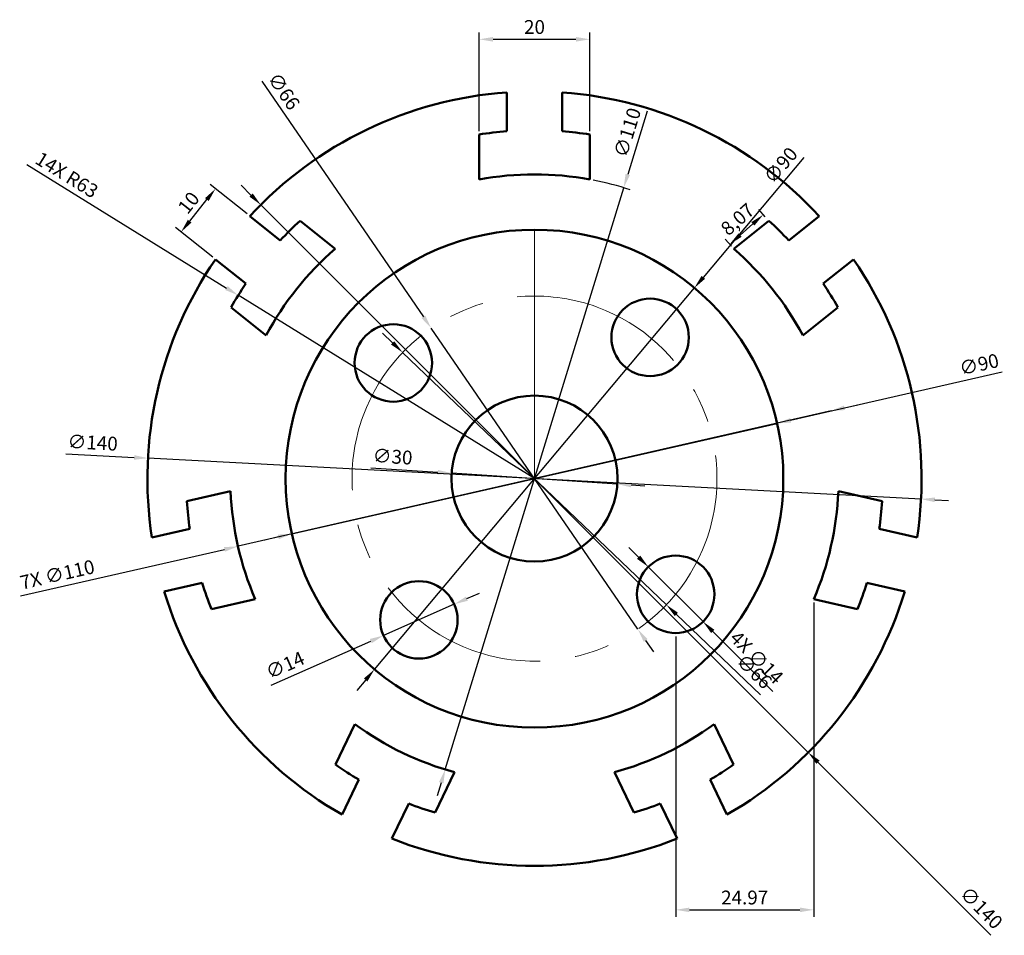
# Model space of a CAD drawing. Units: millimetres. Extents: x 3298 to 3476, y 1660 to 1825.
import ezdxf

# ---------------------------------------------------------------- set-up
doc = ezdxf.new("R2010")
doc.units = ezdxf.units.MM
doc.linetypes.add('CENTER', pattern=[50.8, 31.75, -6.35, 6.35, -6.35])
for name, color, linetype, lineweight in [('M-CNTR', 1, 'CENTER', 18), ('M-CONS', 8, 'Continuous', 13), ('M-DIMS', 2, 'Continuous', 25), ('M-OUTL', 7, 'Continuous', 50)]:
    doc.layers.add(name, color=color, linetype=linetype, lineweight=lineweight)
doc.styles.get("Standard").update_dxf_attribs({"font": 'arial.ttf'})
doc.dimstyles.new('ISO-25', dxfattribs={"dimtxt": 2.5, "dimasz": 2.5, "dimexe": 1.25, "dimexo": 0.625, "dimtad": 1, "dimtxsty": 'Standard', "dimcen": 2.5, "dimadec": 0, "dimazin": 0, "dimtfac": 1, "dimtmove": 0, "dimatfit": 3, "dimfxl": 1, "dimarcsym": 0})

# ---------------------------------------------------------------- blocks, each defined once
blk = doc.blocks.new('*D1')
at = {"layer": 'Defpoints', "color": 0, "transparency": 16777216}
for p in [(3375.77, 1743.34), (3405.71, 1741.37)]:
    blk.add_point(p, dxfattribs=at)
at = {"layer": 'M-DIMS', "color": 0, "lineweight": -2, "transparency": 16777216}
for p, q in [((3361.16, 1744.3), (3373.28, 1743.5)), ((3405.71, 1741.37), (3375.77, 1743.34)), ((3408.2, 1741.21), (3410.69, 1741.05))]:
    blk.add_line(p, q, dxfattribs=at)
at = {"layer": 'M-DIMS', "color": 0, "transparency": 16777216}
for points in [[(3373.3, 1743.92), (3373.25, 1743.09), (3375.77, 1743.34)], [(3408.23, 1741.62), (3408.17, 1740.79), (3405.71, 1741.37)]]:
    blk.add_solid(points, dxfattribs=at)
at = {"layer": 'M-DIMS', "color": 0, "transparency": 16777216, "insert": (3365.06, 1746.02), "char_height": 2.5, "attachment_point": 5, "rotation": 356.242}
blk.add_mtext('∅30', dxfattribs=at)
blk = doc.blocks.new('*D2')
at = {"layer": 'Defpoints', "color": 0, "transparency": 16777216}
for p in [(3434.62, 1752.34), (3346.86, 1732.37)]:
    blk.add_point(p, dxfattribs=at)
at = {"layer": 'M-DIMS', "color": 0, "lineweight": -2, "transparency": 16777216}
for p, q in [((3475.32, 1761.6), (3437.05, 1752.89)), ((3346.86, 1732.37), (3434.62, 1752.34)), ((3344.42, 1731.82), (3341.98, 1731.26))]:
    blk.add_line(p, q, dxfattribs=at)
at = {"layer": 'M-DIMS', "color": 0, "transparency": 16777216}
for points in [[(3436.96, 1753.3), (3437.15, 1752.49), (3434.62, 1752.34)], [(3344.33, 1732.23), (3344.51, 1731.41), (3346.86, 1732.37)]]:
    blk.add_solid(points, dxfattribs=at)
at = {"layer": 'M-DIMS', "color": 0, "transparency": 16777216, "insert": (3471.21, 1762.69), "char_height": 2.5, "attachment_point": 5, "rotation": 12.8166}
blk.add_mtext('∅90', dxfattribs=at)
blk = doc.blocks.new('*D3')
at = {"layer": 'Defpoints', "color": 0, "transparency": 16777216}
for p in [(3376.23, 1719.65), (3363.43, 1714)]:
    blk.add_point(p, dxfattribs=at)
at = {"layer": 'M-DIMS', "color": 0, "lineweight": -2, "transparency": 16777216}
for p, q in [((3378.52, 1720.66), (3380.81, 1721.67)), ((3376.23, 1719.65), (3363.43, 1714)), ((3343.11, 1705.03), (3361.14, 1712.99))]:
    blk.add_line(p, q, dxfattribs=at)
at = {"layer": 'M-DIMS', "color": 0, "transparency": 16777216}
for points in [[(3378.35, 1721.04), (3378.69, 1720.28), (3376.23, 1719.65)], [(3360.97, 1713.37), (3361.31, 1712.61), (3363.43, 1714)]]:
    blk.add_solid(points, dxfattribs=at)
at = {"layer": 'M-DIMS', "color": 0, "transparency": 16777216, "insert": (3345.77, 1708.36), "char_height": 2.5, "attachment_point": 5, "rotation": 23.8194}
blk.add_mtext('∅14', dxfattribs=at)
blk = doc.blocks.new('*D4')
at = {"layer": 'Defpoints', "color": 0, "transparency": 16777216}
for p in [(3372.05, 1769.56), (3409.42, 1715.15)]:
    blk.add_point(p, dxfattribs=at)
at = {"layer": 'M-DIMS', "color": 0, "lineweight": -2, "transparency": 16777216}
for p, q in [((3341.4, 1814.19), (3370.64, 1771.62)), ((3409.42, 1715.15), (3372.05, 1769.56)), ((3410.84, 1713.09), (3412.25, 1711.03))]:
    blk.add_line(p, q, dxfattribs=at)
at = {"layer": 'M-DIMS', "color": 0, "transparency": 16777216}
for points in [[(3370.98, 1771.85), (3370.3, 1771.38), (3372.05, 1769.56)], [(3411.18, 1713.33), (3410.49, 1712.86), (3409.42, 1715.15)]]:
    blk.add_solid(points, dxfattribs=at)
at = {"layer": 'M-DIMS', "color": 0, "transparency": 16777216, "insert": (3345.16, 1812.2), "char_height": 2.5, "attachment_point": 5, "rotation": 304.4835}
blk.add_mtext('∅66', dxfattribs=at)
blk = doc.blocks.new('*D5')
at = {"layer": 'Defpoints', "color": 0, "transparency": 16777216}
for p in [(3406.87, 1794.94), (3374.6, 1689.78)]:
    blk.add_point(p, dxfattribs=at)
at = {"layer": 'M-DIMS', "color": 0, "lineweight": -2, "transparency": 16777216}
for p, q in [((3411.12, 1808.78), (3407.61, 1797.33)), ((3374.6, 1689.78), (3406.87, 1794.94)), ((3373.87, 1687.39), (3373.14, 1685))]:
    blk.add_line(p, q, dxfattribs=at)
blk.add_arc((3390.74, 1742.36), 55, 71.6386, 78.8732, dxfattribs=at)
at = {"layer": 'M-DIMS', "color": 0, "transparency": 16777216}
for points in [[(3407.21, 1797.45), (3408, 1797.2), (3406.87, 1794.94)], [(3373.47, 1687.51), (3374.27, 1687.26), (3374.6, 1689.78)]]:
    blk.add_solid(points, dxfattribs=at)
at = {"layer": 'M-DIMS', "color": 0, "transparency": 16777216, "insert": (3407.85, 1804.83), "char_height": 2.5, "attachment_point": 5, "rotation": 72.9408}
blk.add_mtext('∅110', dxfattribs=at)
blk = doc.blocks.new('*D6')
at = {"layer": 'Defpoints', "color": 0, "transparency": 16777216}
for p in [(3400.74, 1821.77), (3380.74, 1804.56), (3400.74, 1804.56)]:
    blk.add_point(p, dxfattribs=at)
at = {"layer": 'M-DIMS', "color": 0, "lineweight": -2, "transparency": 16777216}
for p, q in [((3380.74, 1805.18), (3380.74, 1823.02)), ((3383.24, 1821.77), (3398.24, 1821.77)), ((3400.74, 1805.18), (3400.74, 1823.02))]:
    blk.add_line(p, q, dxfattribs=at)
at = {"layer": 'M-DIMS', "color": 0, "transparency": 16777216}
for points in [[(3383.24, 1822.19), (3383.24, 1821.35), (3380.74, 1821.77)], [(3398.24, 1822.19), (3398.24, 1821.35), (3400.74, 1821.77)]]:
    blk.add_solid(points, dxfattribs=at)
at = {"layer": 'M-DIMS', "color": 0, "transparency": 16777216, "insert": (3390.74, 1823.67), "char_height": 2.5, "attachment_point": 5}
blk.add_mtext('20', dxfattribs=at)
blk = doc.blocks.new('*D7')
at = {"layer": 'Defpoints', "color": 0, "transparency": 16777216}
for p in [(3432.84, 1789.23), (3426.05, 1784.73), (3426.79, 1783.89)]:
    blk.add_point(p, dxfattribs=at)
at = {"layer": 'M-DIMS', "color": 0, "lineweight": -2, "transparency": 16777216}
for p, q in [((3432.43, 1789.69), (3431.28, 1791)), ((3430.23, 1788.41), (3427.93, 1786.38)), ((3426.37, 1784.36), (3425.22, 1785.67))]:
    blk.add_line(p, q, dxfattribs=at)
at = {"layer": 'M-DIMS', "color": 0, "transparency": 16777216}
for points in [[(3429.95, 1788.72), (3430.51, 1788.1), (3432.11, 1790.06)], [(3427.65, 1786.7), (3428.2, 1786.07), (3426.05, 1784.73)]]:
    blk.add_solid(points, dxfattribs=at)
at = {"layer": 'M-DIMS', "color": 0, "transparency": 16777216, "insert": (3427.67, 1788.99), "char_height": 2.5, "attachment_point": 5, "rotation": 41.3526}
blk.add_mtext('8,07', dxfattribs=at)
blk = doc.blocks.new('*D8')
at = {"layer": 'Defpoints', "color": 0, "transparency": 16777216}
for p in [(3320.84, 1746.05), (3460.64, 1738.66)]:
    blk.add_point(p, dxfattribs=at)
at = {"layer": 'M-DIMS', "color": 0, "lineweight": -2, "transparency": 16777216}
for p, q in [((3305.98, 1746.83), (3318.34, 1746.18)), ((3460.64, 1738.66), (3320.84, 1746.05)), ((3463.14, 1738.53), (3465.63, 1738.4))]:
    blk.add_line(p, q, dxfattribs=at)
at = {"layer": 'M-DIMS', "color": 0, "transparency": 16777216}
for points in [[(3318.36, 1746.6), (3318.32, 1745.77), (3320.84, 1746.05)], [(3463.16, 1738.95), (3463.11, 1738.11), (3460.64, 1738.66)]]:
    blk.add_solid(points, dxfattribs=at)
at = {"layer": 'M-DIMS', "color": 0, "transparency": 16777216, "insert": (3310.82, 1748.55), "char_height": 2.5, "attachment_point": 5, "rotation": 356.9755}
blk.add_mtext('∅140', dxfattribs=at)
blk = doc.blocks.new('RADIAL-T-SLOT-10X20')
for p, q in [((-5, 69.82), (-5, 62.8)), ((5, 69.82), (5, 62.8)), ((-10, 62.2), (-10, 54.08)), ((10, 62.2), (10, 54.08))]:
    blk.add_line(p, q)
for radius, start, end in [(63, 94.5521, 99.1332), (63, 80.8668, 85.4479), (55, 79.5243, 100.4757)]:
    blk.add_arc((0, 0), radius, start, end)
blk = doc.blocks.new('BOLT-HOLE-D14')
blk.add_circle((0, 0), 7)
blk = doc.blocks.new('*D11')
at = {"layer": 'Defpoints', "color": 0, "transparency": 16777216}
for p in [(3333.05, 1794.75), (3339.27, 1789.8), (3333.03, 1781.98)]:
    blk.add_point(p, dxfattribs=at)
at = {"layer": 'M-DIMS', "color": 0, "lineweight": -2, "transparency": 16777216}
for p, q in [((3338.78, 1790.19), (3332.07, 1795.53)), ((3328.38, 1788.89), (3331.49, 1792.8)), ((3332.54, 1782.37), (3325.84, 1787.72))]:
    blk.add_line(p, q, dxfattribs=at)
at = {"layer": 'M-DIMS', "color": 0, "transparency": 16777216}
for points in [[(3331.17, 1793.06), (3331.82, 1792.54), (3333.05, 1794.75)], [(3328.05, 1789.15), (3328.7, 1788.63), (3326.82, 1786.94)]]:
    blk.add_solid(points, dxfattribs=at)
at = {"layer": 'M-DIMS', "color": 0, "transparency": 16777216, "insert": (3328.45, 1792.03), "char_height": 2.5, "attachment_point": 5, "rotation": 51.4286}
blk.add_mtext('10', dxfattribs=at)
blk = doc.blocks.new('*D12')
at = {"layer": 'Defpoints', "color": 0, "transparency": 16777216}
for p in [(3441.24, 1720.57), (3416.27, 1714.45), (3441.24, 1664.41)]:
    blk.add_point(p, dxfattribs=at)
at = {"layer": 'M-DIMS', "color": 0, "lineweight": -2, "transparency": 16777216}
for p, q in [((3441.24, 1719.95), (3441.24, 1663.16)), ((3416.27, 1713.82), (3416.27, 1663.16)), ((3418.77, 1664.41), (3438.74, 1664.41))]:
    blk.add_line(p, q, dxfattribs=at)
at = {"layer": 'M-DIMS', "color": 0, "transparency": 16777216}
for points in [[(3418.77, 1664.82), (3418.77, 1663.99), (3416.27, 1664.41)], [(3438.74, 1664.82), (3438.74, 1663.99), (3441.24, 1664.41)]]:
    blk.add_solid(points, dxfattribs=at)
at = {"layer": 'M-DIMS', "color": 0, "transparency": 16777216, "insert": (3428.75, 1666.31), "char_height": 2.5, "attachment_point": 5}
blk.add_mtext('24.97', dxfattribs=at)
blk = doc.blocks.new('*D13')
at = {"layer": 'Defpoints', "color": 0, "transparency": 16777216}
for p in [(3341.24, 1791.85), (3440.24, 1692.86)]:
    blk.add_point(p, dxfattribs=at)
at = {"layer": 'M-DIMS', "color": 0, "lineweight": -2, "transparency": 16777216}
for p, q in [((3339.47, 1793.62), (3337.7, 1795.39)), ((3341.24, 1791.85), (3440.24, 1692.86)), ((3473.29, 1659.81), (3442, 1691.09))]:
    blk.add_line(p, q, dxfattribs=at)
at = {"layer": 'M-DIMS', "color": 0, "transparency": 16777216}
for points in [[(3339.77, 1793.92), (3339.18, 1793.33), (3341.24, 1791.85)], [(3442.3, 1691.39), (3441.71, 1690.8), (3440.24, 1692.86)]]:
    blk.add_solid(points, dxfattribs=at)
at = {"layer": 'M-DIMS', "color": 0, "transparency": 16777216, "insert": (3471.33, 1664.55), "char_height": 2.5, "attachment_point": 5, "rotation": 315}
blk.add_mtext('∅140', dxfattribs=at)
blk = doc.blocks.new('*D14')
at = {"layer": 'Defpoints', "color": 0, "transparency": 16777216}
for p in [(3337.15, 1775.49), (3390.74, 1742.36)]:
    blk.add_point(p, dxfattribs=at)
at = {"layer": 'M-DIMS', "color": 0, "lineweight": -2, "transparency": 16777216}
for p, q in [((3298.92, 1799.13), (3335.03, 1776.8)), ((3390.74, 1742.36), (3337.15, 1775.49))]:
    blk.add_line(p, q, dxfattribs=at)
at = {"layer": 'M-DIMS', "color": 0, "transparency": 16777216}
blk.add_solid([(3335.25, 1777.16), (3334.81, 1776.45), (3337.15, 1775.49)], dxfattribs=at)
at = {"layer": 'M-DIMS', "color": 0, "transparency": 16777216, "insert": (3306, 1796.98), "char_height": 2.5, "attachment_point": 5, "rotation": 328.2712}
blk.add_mtext('14X R63', dxfattribs=at)
blk = doc.blocks.new('*D15')
at = {"layer": 'Defpoints', "color": 0, "transparency": 16777216}
for p in [(3444.36, 1754.6), (3337.12, 1730.12)]:
    blk.add_point(p, dxfattribs=at)
at = {"layer": 'M-DIMS', "color": 0, "lineweight": -2, "transparency": 16777216}
for p, q in [((3446.8, 1755.15), (3449.23, 1755.71)), ((3444.36, 1754.6), (3337.12, 1730.12)), ((3297.78, 1721.14), (3334.68, 1729.56))]:
    blk.add_line(p, q, dxfattribs=at)
at = {"layer": 'M-DIMS', "color": 0, "transparency": 16777216}
for points in [[(3446.7, 1755.56), (3446.89, 1754.75), (3444.36, 1754.6)], [(3334.59, 1729.97), (3334.77, 1729.15), (3337.12, 1730.12)]]:
    blk.add_solid(points, dxfattribs=at)
at = {"layer": 'M-DIMS', "color": 0, "transparency": 16777216, "insert": (3304.51, 1724.7), "char_height": 2.5, "attachment_point": 5, "rotation": 12.8576}
blk.add_mtext('7X ∅110', dxfattribs=at)
blk = doc.blocks.new('*D16')
at = {"layer": 'Defpoints', "color": 0, "transparency": 16777216}
for p in [(3419.66, 1776.83), (3361.81, 1707.88)]:
    blk.add_point(p, dxfattribs=at)
at = {"layer": 'M-DIMS', "color": 0, "lineweight": -2, "transparency": 16777216}
for p, q in [((3439.44, 1800.4), (3421.27, 1778.74)), ((3361.81, 1707.88), (3419.66, 1776.83)), ((3360.21, 1705.97), (3358.6, 1704.05))]:
    blk.add_line(p, q, dxfattribs=at)
at = {"layer": 'M-DIMS', "color": 0, "transparency": 16777216}
for points in [[(3420.95, 1779.01), (3421.59, 1778.48), (3419.66, 1776.83)], [(3359.89, 1706.24), (3360.52, 1705.7), (3361.81, 1707.88)]]:
    blk.add_solid(points, dxfattribs=at)
at = {"layer": 'M-DIMS', "color": 0, "transparency": 16777216, "insert": (3435.51, 1798.78), "char_height": 2.5, "attachment_point": 5, "rotation": 50.0003}
blk.add_mtext('∅90', dxfattribs=at)
blk = doc.blocks.new('*D17')
at = {"layer": 'Defpoints', "color": 0, "transparency": 16777216}
for p in [(3366.89, 1765.17), (3414.59, 1719.55)]:
    blk.add_point(p, dxfattribs=at)
at = {"layer": 'M-DIMS', "color": 0, "lineweight": -2, "transparency": 16777216}
for p, q in [((3365.08, 1766.89), (3363.28, 1768.62)), ((3366.89, 1765.17), (3414.59, 1719.55)), ((3431.62, 1703.25), (3416.39, 1717.82))]:
    blk.add_line(p, q, dxfattribs=at)
at = {"layer": 'M-DIMS', "color": 0, "transparency": 16777216}
for points in [[(3365.37, 1767.2), (3364.8, 1766.59), (3366.89, 1765.17)], [(3416.68, 1718.12), (3416.1, 1717.52), (3414.59, 1719.55)]]:
    blk.add_solid(points, dxfattribs=at)
at = {"layer": 'M-DIMS', "color": 0, "transparency": 16777216, "insert": (3430.26, 1707.28), "char_height": 2.5, "attachment_point": 5, "rotation": 316.2732}
blk.add_mtext('∅66', dxfattribs=at)
blk = doc.blocks.new('*D18')
at = {"layer": 'Defpoints', "color": 0, "transparency": 16777216}
for p in [(3411.32, 1726.4), (3421.22, 1716.5)]:
    blk.add_point(p, dxfattribs=at)
at = {"layer": 'M-DIMS', "color": 0, "lineweight": -2, "transparency": 16777216}
for p, q in [((3409.55, 1728.16), (3407.78, 1729.93)), ((3411.32, 1726.4), (3421.22, 1716.5)), ((3433.87, 1703.86), (3422.99, 1714.73))]:
    blk.add_line(p, q, dxfattribs=at)
at = {"layer": 'M-DIMS', "color": 0, "transparency": 16777216}
for points in [[(3409.85, 1728.46), (3409.26, 1727.87), (3411.32, 1726.4)], [(3423.28, 1715.03), (3422.69, 1714.44), (3421.22, 1716.5)]]:
    blk.add_solid(points, dxfattribs=at)
at = {"layer": 'M-DIMS', "color": 0, "transparency": 16777216, "insert": (3430.7, 1709.81), "char_height": 2.5, "attachment_point": 5, "rotation": 315.0106}
blk.add_mtext('4X ∅14', dxfattribs=at)

msp = doc.modelspace()

# ---------------------------------------------------------------- linework, layer by layer
at = {"layer": 'M-CNTR'}
msp.add_circle((3390.738, 1742.356), 33, dxfattribs=at)
at = {"layer": 'M-CONS'}
for p, q in [((3426.787, 1783.895), (3433.042, 1788.883)), ((3390.738, 1742.356), (3390.738, 1787.356)), ((3323.78, 1721.945), (3324.427, 1722.093))]:
    msp.add_line(p, q, dxfattribs=at)
at = {"layer": 'M-OUTL'}
for radius in [45, 15]:
    msp.add_circle((3390.738, 1742.356), radius, dxfattribs=at)
for start, end in [(94.09604, 137.33253), (42.66747, 85.90396), (145.52462, 188.7611), (351.2389, 34.47538), (196.95319, 240.18967), (299.81033, 343.04681), (248.38176, 291.61824)]:
    msp.add_arc((3390.738, 1742.356), 70, start, end, dxfattribs=at)

# ---------------------------------------------------------------- block references
for name, p in [('RADIAL-T-SLOT-10X20', (3390.738, 1742.356)), ('BOLT-HOLE-D14', (3411.646, 1767.888)), ('BOLT-HOLE-D14', (3365.206, 1763.264)), ('BOLT-HOLE-D14', (3416.27, 1721.448)), ('BOLT-HOLE-D14', (3369.83, 1716.824))]:
    msp.add_blockref(name, p, dxfattribs=at)
for rotation in [51.4285714285701, 308.5714285714283, 102.8571428571406, 257.1428571428524, 154.2857142857166, 205.7142857142829]:
    msp.add_blockref('RADIAL-T-SLOT-10X20', (3390.738, 1742.356), dxfattribs=dict(at, rotation=rotation))

# ---------------------------------------------------------------- dimensions: what is measured, and where the dimension line sits
at = {"layer": 'M-DIMS'}
for base, p1, p2, override, picture, middle in [((3400.738, 1821.77), (3380.738, 1804.557), (3400.738, 1804.557), {"dimclrd": 0, "dimclre": 0, "dimclrt": 0}, '*D6', (3390.738, 1823.671)), ((3441.24, 1664.406), (3416.27, 1714.448), (3441.24, 1720.572), {"dimdec": 2, "dimlfac": 1, "dimrnd": 0, "dimzin": 0, "dimdsep": 46, "dimlunit": 2}, '*D12', (3428.755, 1666.308))]:
    dim = msp.add_linear_dim(base=base, p1=p1, p2=p2, dimstyle='ISO-25', override=override, dxfattribs=at)
    dim.commit()
    dim.dimension.update_dxf_attribs({"geometry": picture, "text_midpoint": middle})
for p1, p2, override, picture, middle in [((3409.422, 1715.155), (3372.054, 1769.558), {"dimclrd": 0, "dimclre": 0, "dimclrt": 0}, '*D4', (3343.533, 1811.081)), ((3361.813, 1707.884), (3419.663, 1776.828), {"dimdec": 0, "dimlfac": 1, "dimrnd": 0, "dimzin": 0, "dimdsep": 46, "dimlunit": 2}, '*D16', (3437.018, 1797.512)), ((3341.24, 1791.854), (3440.235, 1692.859), {"dimdec": 0, "dimlfac": 1, "dimrnd": 0, "dimzin": 0, "dimdsep": 46, "dimlunit": 2}, '*D13', (3469.934, 1663.16)), ((3366.891, 1765.166), (3414.585, 1719.546), {"dimdec": 0, "dimlfac": 1, "dimrnd": 0, "dimzin": 0, "dimdsep": 46, "dimlunit": 2}, '*D17', (3428.894, 1705.86)), ((3346.859, 1732.374), (3434.617, 1752.339), {"dimclrd": 0, "dimclre": 0, "dimclrt": 0}, '*D2', (3471.647, 1760.763)), ((3460.64, 1738.663), (3320.835, 1746.05), {"dimclrd": 0, "dimclre": 0, "dimclrt": 0}, '*D8', (3310.712, 1746.584)), ((3405.706, 1741.373), (3375.77, 1743.339), {"dimclrd": 0, "dimclre": 0, "dimclrt": 0}, '*D1', (3364.927, 1744.051)), ((3376.234, 1719.651), (3363.427, 1713.997), {"dimclrd": 0, "dimclre": 0, "dimclrt": 0}, '*D3', (3346.563, 1706.553))]:
    dim = msp.add_diameter_dim_2p(p1=p1, p2=p2, dimstyle='ISO-25', override=override, dxfattribs=at)
    dim.commit()
    dim.dimension.update_dxf_attribs({"geometry": picture, "text_midpoint": middle, "dimtype": 163})
dim = msp.add_diameter_dim_2p(p1=(3374.603, 1689.776), p2=(3406.873, 1794.936), dimstyle='ISO-25', override={"dimclrd": 0, "dimclre": 0, "dimclrt": 0}, dxfattribs=at)
dim.commit()
dim.dimension.update_dxf_attribs({"geometry": '*D5', "text_midpoint": (3407.846, 1804.828)})
dim = msp.add_radius_dim(center=(3390.738, 1742.356), mpoint=(3337.153, 1775.488), text='14X <>', dimstyle='ISO-25', override={"dimdec": 0, "dimlfac": 1, "dimrnd": 0, "dimzin": 0, "dimdsep": 46, "dimlunit": 2}, dxfattribs=at)
dim.commit()
dim.dimension.update_dxf_attribs({"geometry": '*D14', "text_midpoint": (3305.003, 1795.367), "dimtype": 164})
dim = msp.add_linear_dim(base=(3333.051, 1794.755), p1=(3333.032, 1781.98), p2=(3339.267, 1789.798), angle=51.42857, dimstyle='ISO-25', override={"dimdec": 0, "dimlfac": 1, "dimrnd": 0, "dimzin": 0, "dimdsep": 46, "dimlunit": 2}, dxfattribs=at)
dim.commit()
dim.dimension.update_dxf_attribs({"geometry": '*D11', "text_midpoint": (3328.447, 1792.031)})
dim = msp.add_aligned_dim(p1=(3432.844, 1789.226), p2=(3426.787, 1783.895), distance=-1.116, dimstyle='ISO-25', override={"dimclrd": 0, "dimclre": 0, "dimclrt": 0}, dxfattribs=at)
dim.commit()
dim.dimension.update_dxf_attribs({"geometry": '*D7', "text_midpoint": (3427.673, 1788.995)})
for p1, p2, text, picture, middle in [((3444.359, 1754.595), (3337.117, 1730.117), '7X <>', '*D15', (3304.944, 1722.774)), ((3411.319, 1726.397), (3421.22, 1716.5), '4X <>', '*D18', (3429.311, 1708.412))]:
    dim = msp.add_diameter_dim_2p(p1=p1, p2=p2, text=text, dimstyle='ISO-25', override={"dimdec": 0, "dimlfac": 1, "dimrnd": 0, "dimzin": 0, "dimdsep": 46, "dimlunit": 2}, dxfattribs=at)
    dim.commit()
    dim.dimension.update_dxf_attribs({"geometry": picture, "text_midpoint": middle, "dimtype": 163})

doc.saveas('drawing.dxf')
